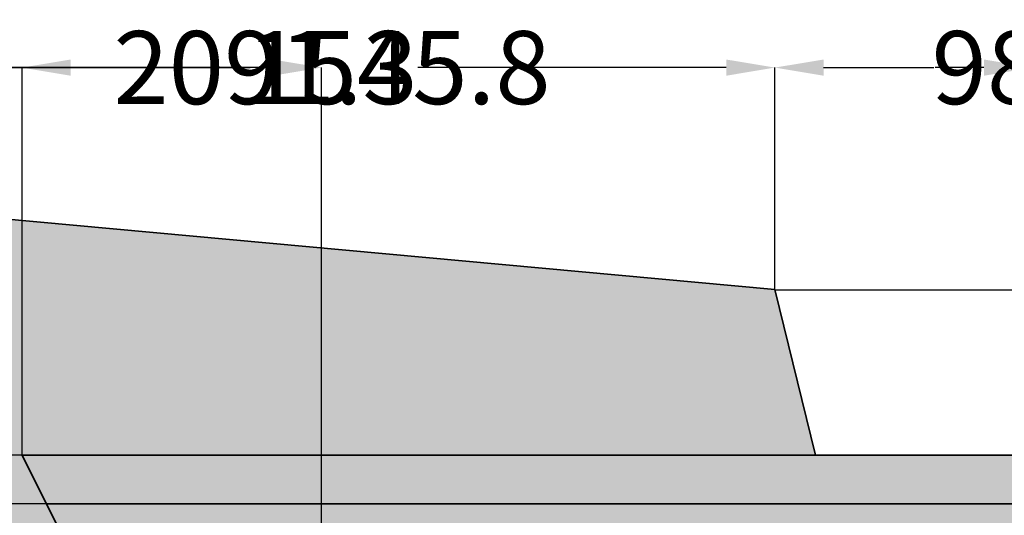
# Model space of a CAD drawing. Units: millimetres. Extents: x -504 to 6314, y 1290 to 4335.
# Tile 5 of 9: x 1774 to 3796, y 3317 to 4335. Entities that reach past the tile are written whole.
import ezdxf

# ---------------------------------------------------------------- set-up
doc = ezdxf.new("R2010")
doc.units = ezdxf.units.MM
doc.header["$MEASUREMENT"] = 0
for name, color, linetype, lineweight in [('A-ANNO-DIMS', 2, 'Continuous', 18), ('A-ELEV', 7, 'Continuous', 35), ('A-ELEV-PATT', 8, 'Continuous', 13)]:
    doc.layers.add(name, color=color, linetype=linetype, lineweight=lineweight)
doc.styles.get("Standard").update_dxf_attribs({"font": 'arial.ttf'})
doc.dimstyles.get("Standard").update_dxf_attribs({"dimtxt": 150, "dimasz": 100, "dimexe": 0.18, "dimexo": 0.0625, "dimgap": 0.09, "dimtad": 0, "dimtih": 1, "dimtoh": 1, "dimdec": 0, "dimzin": 0, "dimdsep": 46, "dimtxsty": 'Standard', "dimcen": 0.09, "dimadec": 0, "dimazin": 0, "dimtfac": 1, "dimtdec": 0, "dimtofl": 0, "dimtmove": 0, "dimatfit": 3, "dimfxl": 1, "dimtolj": 1, "dimtzin": 0, "dimarcsym": 0})

# ---------------------------------------------------------------- blocks, each defined once
blk = doc.blocks.new('*D4')
at = {"layer": 'A-ANNO-DIMS', "color": 0, "lineweight": -2, "transparency": 16777216}
for p, q in [((1233.2, 3972.8), (1233.2, 4237)), ((1333.2, 4236.8), (1966.1, 4236.8)), ((3224.5, 4236.8), (2591.5, 4236.8)), ((3324.5, 3780.7), (3324.5, 4237))]:
    blk.add_line(p, q, dxfattribs=at)
at = {"layer": 'A-ANNO-DIMS', "color": 0, "transparency": 16777216}
for points in [[(1333.2, 4253.4), (1333.2, 4220.1), (1233.2, 4236.8)], [(3224.5, 4253.4), (3224.5, 4220.1), (3324.5, 4236.8)]]:
    blk.add_solid(points, dxfattribs=at)
at = {"layer": 'Defpoints', "color": 0, "transparency": 16777216}
for p in [(3324.5, 4236.8), (1233.2, 3972.8), (3324.5, 3780.6)]:
    blk.add_point(p, dxfattribs=at)
at = {"layer": 'A-ANNO-DIMS', "color": 0, "transparency": 16777216, "insert": (2278.8, 4236.8), "char_height": 150, "attachment_point": 5}
blk.add_mtext('\\A1;2091.3', dxfattribs=at)
blk = doc.blocks.new('*D6')
at = {"layer": 'A-ANNO-DIMS', "color": 0, "lineweight": -2, "transparency": 16777216}
for p, q in [((72.8, 1652.2), (72.8, 4237)), ((172.8, 4236.8), (920.4, 4236.8)), ((2293.5, 4236.8), (1545.9, 4236.8)), ((2393.5, 1652.2), (2393.5, 4237))]:
    blk.add_line(p, q, dxfattribs=at)
at = {"layer": 'A-ANNO-DIMS', "color": 0, "transparency": 16777216}
for points in [[(172.8, 4253.4), (172.8, 4220.1), (72.8, 4236.8)], [(2293.5, 4253.4), (2293.5, 4220.1), (2393.5, 4236.8)]]:
    blk.add_solid(points, dxfattribs=at)
at = {"layer": 'Defpoints', "color": 0, "transparency": 16777216}
for p in [(2393.5, 4236.8), (72.8, 1652.1), (2393.5, 1652.1)]:
    blk.add_point(p, dxfattribs=at)
at = {"layer": 'A-ANNO-DIMS', "color": 0, "transparency": 16777216, "insert": (1233.2, 4236.8), "char_height": 150, "attachment_point": 5}
blk.add_mtext('\\A1;2320.7', dxfattribs=at)
blk = doc.blocks.new('*D21')
at = {"layer": 'A-ANNO-DIMS', "color": 0, "lineweight": -2, "transparency": 16777216}
for p, q in [((1778.7, 3440.7), (1778.7, 4237)), ((1878.7, 4236.8), (2247.1, 4236.8)), ((3224.5, 4236.8), (2856.1, 4236.8)), ((3324.5, 3780.7), (3324.5, 4237))]:
    blk.add_line(p, q, dxfattribs=at)
at = {"layer": 'A-ANNO-DIMS', "color": 0, "transparency": 16777216}
for points in [[(1878.7, 4253.4), (1878.7, 4220.1), (1778.7, 4236.8)], [(3224.5, 4253.4), (3224.5, 4220.1), (3324.5, 4236.8)]]:
    blk.add_solid(points, dxfattribs=at)
at = {"layer": 'Defpoints', "color": 0, "transparency": 16777216}
for p in [(3324.5, 4236.8), (3324.5, 3780.6), (1778.7, 3440.7)]:
    blk.add_point(p, dxfattribs=at)
at = {"layer": 'A-ANNO-DIMS', "color": 0, "transparency": 16777216, "insert": (2551.6, 4236.8), "char_height": 150, "attachment_point": 5}
blk.add_mtext('\\A1;1545.8', dxfattribs=at)
blk = doc.blocks.new('*D22')
at = {"layer": 'A-ANNO-DIMS', "color": 0, "lineweight": -2, "transparency": 16777216}
for p, q in [((3324.5, 3780.7), (3324.5, 4237)), ((3424.5, 4236.8), (3651, 4236.8)), ((4208.6, 4236.8), (3982, 4236.8)), ((4308.6, 3440.7), (4308.6, 4237))]:
    blk.add_line(p, q, dxfattribs=at)
at = {"layer": 'A-ANNO-DIMS', "color": 0, "transparency": 16777216}
for points in [[(3424.5, 4253.4), (3424.5, 4220.1), (3324.5, 4236.8)], [(4208.6, 4253.4), (4208.6, 4220.1), (4308.6, 4236.8)]]:
    blk.add_solid(points, dxfattribs=at)
at = {"layer": 'Defpoints', "color": 0, "transparency": 16777216}
for p in [(4308.6, 4236.8), (3324.5, 3780.6), (4308.6, 3440.7)]:
    blk.add_point(p, dxfattribs=at)
at = {"layer": 'A-ANNO-DIMS', "color": 0, "transparency": 16777216, "insert": (3816.5, 4236.8), "char_height": 150, "attachment_point": 5}
blk.add_mtext('\\A1;984', dxfattribs=at)
blk = doc.blocks.new('*D24')
at = {"layer": 'A-ANNO-DIMS', "color": 0, "lineweight": -2, "transparency": 16777216}
for p, q in [((5588.8, 3780.6), (5588.8, 3880.6)), ((5588.8, 3880.6), (5688.8, 3880.6)), ((3324.5, 3780.6), (5589, 3780.6)), ((5588.8, 3540.7), (5588.8, 3680.6)), ((4308.6, 3440.7), (5589, 3440.7))]:
    blk.add_line(p, q, dxfattribs=at)
at = {"layer": 'A-ANNO-DIMS', "color": 0, "transparency": 16777216}
for points in [[(5572.1, 3680.6), (5605.5, 3680.6), (5588.8, 3780.6)], [(5572.1, 3540.7), (5605.5, 3540.7), (5588.8, 3440.7)]]:
    blk.add_solid(points, dxfattribs=at)
at = {"layer": 'Defpoints', "color": 0, "transparency": 16777216}
for p in [(3324.5, 3780.6), (5588.8, 3780.6), (4308.6, 3440.7)]:
    blk.add_point(p, dxfattribs=at)
at = {"layer": 'A-ANNO-DIMS', "color": 0, "transparency": 16777216, "insert": (5999.9, 3880.6), "char_height": 150, "attachment_point": 5}
blk.add_mtext('\\A1;339.94', dxfattribs=at)
blk = doc.blocks.new('*D28')
at = {"layer": 'A-ANNO-DIMS', "color": 0, "lineweight": -2, "transparency": 16777216}
for p, q in [((-191.2, 3540.7), (-191.2, 3640.7)), ((-191.2, 3640.7), (-91.2, 3640.7)), ((4308.5, 3440.7), (-191.3, 3440.7)), ((4304.4, 3340.7), (-191.3, 3340.7)), ((-191.2, 3240.7), (-191.2, 3140.7))]:
    blk.add_line(p, q, dxfattribs=at)
at = {"layer": 'A-ANNO-DIMS', "color": 0, "transparency": 16777216}
for points in [[(-207.8, 3540.7), (-174.5, 3540.7), (-191.2, 3440.7)], [(-207.8, 3240.7), (-174.5, 3240.7), (-191.2, 3340.7)]]:
    blk.add_solid(points, dxfattribs=at)
at = {"layer": 'Defpoints', "color": 0, "transparency": 16777216}
for p in [(-191.2, 3440.7), (4308.6, 3440.7), (4304.5, 3340.7)]:
    blk.add_point(p, dxfattribs=at)
at = {"layer": 'A-ANNO-DIMS', "color": 0, "transparency": 16777216, "insert": (67.3, 3640.7), "char_height": 150, "attachment_point": 5}
blk.add_mtext('\\A1;100', dxfattribs=at)
blk = doc.blocks.new('*D33')
at = {"layer": 'A-ANNO-DIMS', "color": 0, "lineweight": -2, "transparency": 16777216}
for p, q in [((-191.2, 3315.7), (-191.2, 3415.7)), ((-191.2, 3415.7), (-91.2, 3415.7)), ((2963.6, 3215.7), (-191.3, 3215.7)), ((2963.6, 3115.7), (-191.3, 3115.7)), ((-191.2, 3015.7), (-191.2, 2915.7))]:
    blk.add_line(p, q, dxfattribs=at)
at = {"layer": 'A-ANNO-DIMS', "color": 0, "transparency": 16777216}
for points in [[(-207.8, 3315.7), (-174.5, 3315.7), (-191.2, 3215.7)], [(-207.8, 3015.7), (-174.5, 3015.7), (-191.2, 3115.7)]]:
    blk.add_solid(points, dxfattribs=at)
at = {"layer": 'Defpoints', "color": 0, "transparency": 16777216}
for p in [(-191.2, 3215.7), (2963.6, 3215.7), (2963.6, 3115.7)]:
    blk.add_point(p, dxfattribs=at)
at = {"layer": 'A-ANNO-DIMS', "color": 0, "transparency": 16777216, "insert": (67.3, 3415.7), "char_height": 150, "attachment_point": 5}
blk.add_mtext('\\A1;100', dxfattribs=at)
blk = doc.blocks.new('*D34')
at = {"layer": 'A-ANNO-DIMS', "color": 0, "lineweight": -2, "transparency": 16777216}
for p, q in [((-191.2, 3390.7), (-191.2, 3490.7)), ((-191.2, 3490.7), (-91.2, 3490.7)), ((2963.6, 3290.7), (-191.3, 3290.7)), ((2963.6, 3215.7), (-191.3, 3215.7)), ((-191.2, 3115.7), (-191.2, 3015.7))]:
    blk.add_line(p, q, dxfattribs=at)
at = {"layer": 'A-ANNO-DIMS', "color": 0, "transparency": 16777216}
for points in [[(-207.8, 3390.7), (-174.5, 3390.7), (-191.2, 3290.7)], [(-207.8, 3115.7), (-174.5, 3115.7), (-191.2, 3215.7)]]:
    blk.add_solid(points, dxfattribs=at)
at = {"layer": 'Defpoints', "color": 0, "transparency": 16777216}
for p in [(-191.2, 3290.7), (2963.6, 3290.7), (2963.6, 3215.7)]:
    blk.add_point(p, dxfattribs=at)
at = {"layer": 'A-ANNO-DIMS', "color": 0, "transparency": 16777216, "insert": (16.3, 3490.7), "char_height": 150, "attachment_point": 5}
blk.add_mtext('\\A1;75', dxfattribs=at)
blk = doc.blocks.new('*D66')
at = {"layer": 'A-ANNO-DIMS', "color": 0, "lineweight": -2, "transparency": 16777216}
for p, q in [((3753.7, 4236.8), (3653.7, 4236.8)), ((3853.7, 1932.9), (3853.7, 4237)), ((3992.1, 1982.9), (3992.1, 4237)), ((4092.1, 4236.8), (4192.1, 4236.8))]:
    blk.add_line(p, q, dxfattribs=at)
at = {"layer": 'A-ANNO-DIMS', "color": 0, "transparency": 16777216}
for points in [[(3753.7, 4253.4), (3753.7, 4220.1), (3853.7, 4236.8)], [(4092.1, 4253.4), (4092.1, 4220.1), (3992.1, 4236.8)]]:
    blk.add_solid(points, dxfattribs=at)
at = {"layer": 'Defpoints', "color": 0, "transparency": 16777216}
for p in [(3992.1, 4236.8), (3992.1, 1982.8), (3853.7, 1932.8)]:
    blk.add_point(p, dxfattribs=at)
at = {"layer": 'A-ANNO-DIMS', "color": 0, "transparency": 16777216, "insert": (4496.6, 4236.8), "char_height": 150, "attachment_point": 5}
blk.add_mtext('\\A1;138.38', dxfattribs=at)

msp = doc.modelspace()

# ---------------------------------------------------------------- hatches: boundary and pattern name
at = {"layer": 'A-ELEV-PATT'}
for points in [[(3324.48, 3780.626), (1233.163, 3972.781), (72.835, 1652.125), (2393.491, 1652.125), (2355.991, 1727.125), (138.286, 1727.125), (1247.138, 3944.83), (2393.491, 1652.125), (2840.705, 1652.125), (2403.888, 2525.758), (2236.182, 2525.758), (2186.182, 2625.758), (2309.166, 2625.758), (1976.702, 3290.687), (1853.718, 3290.687), (1778.718, 3440.687), (3407.797, 3440.687)], [(4308.57, 3440.687), (3929.687, 3440.687), (3407.797, 3440.687), (1778.718, 3440.687), (1828.718, 3340.687), (3407.797, 3340.687), (3929.687, 3340.687), (4304.463, 3340.687), (5081.168, 3138.941), (5082.876, 3139.564), (5082.876, 3239.564)]]:
    msp.add_hatch(color=256, dxfattribs=at).paths.add_polyline_path(points)
h = msp.add_hatch(dxfattribs=at)
h.set_pattern_fill('ANSI36', color=256, scale=200, angle=135, style=0)
h.paths.add_polyline_path([(3324.48, 3780.626), (1233.163, 3972.781), (72.835, 1652.125), (2393.491, 1652.125), (2355.991, 1727.125), (138.286, 1727.125), (1247.138, 3944.83), (2393.491, 1652.125), (2840.705, 1652.125), (2403.888, 2525.758), (2236.182, 2525.758), (2186.182, 2625.758), (2309.166, 2625.758), (1976.702, 3290.687), (1853.718, 3290.687), (1778.718, 3440.687), (3407.797, 3440.687)])
h = msp.add_hatch(dxfattribs=at)
h.set_pattern_fill('AR-CONC', color=256, scale=10, style=0)
h.set_pattern_definition([(50, (0, 0), (71.726, -6.2752), [7.5, -82.5]), (355, (0, 0), (-13.8751, 75.2192), [6, -66]), (100.4514, (5.98, -0.52), (57.8509, 68.944), [6.374, -70.1142]), (46.1842, (0, 20), (106.7241, -16.5519), [11.25, -123.75]), (96.6356, (8.89, 18.62), (93.4662, 97.4119), [9.561, -105.1714]), (351.1842, (0, 20), (93.4662, 97.4119), [9, -99]), (21, (10, 15), (59.6907, -40.2619), [7.5, -82.5]), (326, (10, 15), (24.3315, 72.515), [6, -66]), (71.4514, (14.974, 11.645), (84.0222, 32.2531), [6.374, -70.1142]), (37.5, (0, 0), (1.21599, 33.28939), [0, -65.2, 0, -67, 0, -66.25]), (7.5, (0, 0), (26.30695, 39.44117), [0, -38.2, 0, -63.7, 0, -25.25]), (327.5, (-22.3, 0), (53.38224, -2.25549), [0, -25, 0, -78, 0, -103.5]), (317.5, (-32.3, 0), (58.3186, 10.0105), [0, -32.5, 0, -51.8, 0, -73.5])])
h.paths.add_polyline_path([(4308.57, 3440.687), (3929.687, 3440.687), (3407.797, 3440.687), (1778.718, 3440.687), (1828.718, 3340.687), (3407.797, 3340.687), (3929.687, 3340.687), (4304.463, 3340.687), (5081.168, 3138.941), (5082.876, 3139.564), (5082.876, 3239.564)])
h.paths.add_polyline_path([(4260.021, 2625.758), (3929.687, 2625.758), (3407.797, 2625.758), (2186.182, 2625.758), (2223.682, 2550.758), (3407.797, 2550.758), (3929.687, 2550.758), (4250.093, 2550.758), (5324.792, 2261.16), (5324.792, 2338.836)])
h = msp.add_hatch(color=256, dxfattribs=at)
h.paths.add_polyline_path([(4304.463, 3340.687), (3929.687, 3340.687), (3407.797, 3340.687), (1828.718, 3340.687), (1853.718, 3290.687), (1976.702, 3290.687), (2309.166, 2625.758), (2353.888, 2625.758), (2021.423, 3290.687), (2963.634, 3290.687), (2963.634, 3265.687), (3407.797, 3265.687), (3768.634, 3265.687), (3768.634, 3290.687), (3793.634, 3290.687), (3793.634, 2625.758), (3818.634, 2625.758), (3818.634, 3290.687), (3929.687, 3290.687), (4198.634, 3290.687), (4473.634, 3219.257), (4473.634, 2568.197), (4498.634, 2561.46), (4498.634, 3167.307), (4673.634, 3167.307), (4923.634, 3102.371), (4923.634, 3081.487), (5081.168, 3138.941)])
h.paths.add_polyline_path([(3768.634, 3240.687), (3407.797, 3240.687), (2963.634, 3240.687), (2963.634, 3290.687), (2913.634, 3290.687), (2913.634, 2625.758), (2963.634, 2625.758), (2963.634, 3215.687), (3407.797, 3215.687), (3768.634, 3215.687)], flags=17)

# ---------------------------------------------------------------- linework, layer by layer
at = {"layer": 'A-ELEV'}
for p, q in [((1233.163, 3972.781), (3324.48, 3780.626)), ((3324.48, 3780.626), (3407.797, 3440.687)), ((3407.797, 3440.687), (1778.718, 3440.687)), ((1778.718, 3440.687), (1853.718, 3290.687)), ((3407.797, 3440.687), (3929.687, 3440.687)), ((3407.797, 3340.687), (1828.718, 3340.687)), ((3407.797, 3340.687), (3929.687, 3340.687))]:
    msp.add_line(p, q, dxfattribs=at)

# ---------------------------------------------------------------- dimensions: what is measured, and where the dimension line sits
at = {"layer": 'A-ANNO-DIMS'}
for base, p1, p2, override, picture, middle in [((2393.491, 4236.781), (72.835, 1652.125), (2393.491, 1652.125), {"dimdec": 1, "dimlfac": 1, "dimrnd": 0, "dimzin": 0, "dimdsep": 46, "dimlunit": 2}, '*D6', (1233.163, 4236.781)), ((3324.48, 4236.781), (1233.163, 3972.781), (3324.48, 3780.626), {"dimdec": 1, "dimlfac": 1, "dimrnd": 0, "dimzin": 0, "dimdsep": 46, "dimlunit": 2}, '*D4', (2278.822, 4236.781)), ((3324.48, 4236.781), (1778.718, 3440.687), (3324.48, 3780.626), {"dimdec": 1, "dimlfac": 1, "dimrnd": 0, "dimzin": 0, "dimdsep": 46, "dimlunit": 2}, '*D21', (2551.599, 4236.781)), ((4308.57, 4236.781), (3324.48, 3780.626), (4308.57, 3440.687), {"dimdec": 0, "dimlfac": 1, "dimrnd": 0, "dimzin": 0, "dimdsep": 46, "dimlunit": 2}, '*D22', (3816.525, 4236.781)), ((3992.087, 4236.781), (3853.708, 1932.831), (3992.087, 1982.831), {"dimdec": 2, "dimlfac": 1, "dimrnd": 0, "dimzin": 0, "dimdsep": 46, "dimlunit": 2}, '*D66', (4496.628, 4236.781))]:
    dim = msp.add_linear_dim(base=base, p1=p1, p2=p2, dimstyle='Standard', override=override, dxfattribs=at)
    dim.commit()
    dim.dimension.update_dxf_attribs({"geometry": picture, "text_midpoint": middle})
for base, p1, p2, override, picture, middle in [((5588.792, 3780.626), (4308.57, 3440.687), (3324.48, 3780.626), {"dimdec": 2, "dimlfac": 1, "dimrnd": 0, "dimzin": 0, "dimdsep": 46, "dimlunit": 2}, '*D24', (5999.881, 3880.626)), ((-191.165, 3440.687), (4304.463, 3340.687), (4308.57, 3440.687), {"dimdec": 0, "dimlfac": 1, "dimrnd": 0, "dimzin": 0, "dimdsep": 46, "dimlunit": 2}, '*D28', (67.315, 3640.687)), ((-191.165, 3290.687), (2963.634, 3215.687), (2963.634, 3290.687), {"dimdec": 0, "dimlfac": 1, "dimrnd": 0, "dimzin": 0, "dimdsep": 46, "dimlunit": 2}, '*D34', (16.309, 3490.687)), ((-191.165, 3215.687), (2963.634, 3115.687), (2963.634, 3215.687), {"dimdec": 0, "dimlfac": 1, "dimrnd": 0, "dimzin": 0, "dimdsep": 46, "dimlunit": 2}, '*D33', (67.315, 3415.687))]:
    dim = msp.add_linear_dim(base=base, p1=p1, p2=p2, angle=90, dimstyle='Standard', override=override, dxfattribs=at)
    dim.commit()
    dim.dimension.update_dxf_attribs({"geometry": picture, "text_midpoint": middle})

doc.saveas('drawing.dxf')
